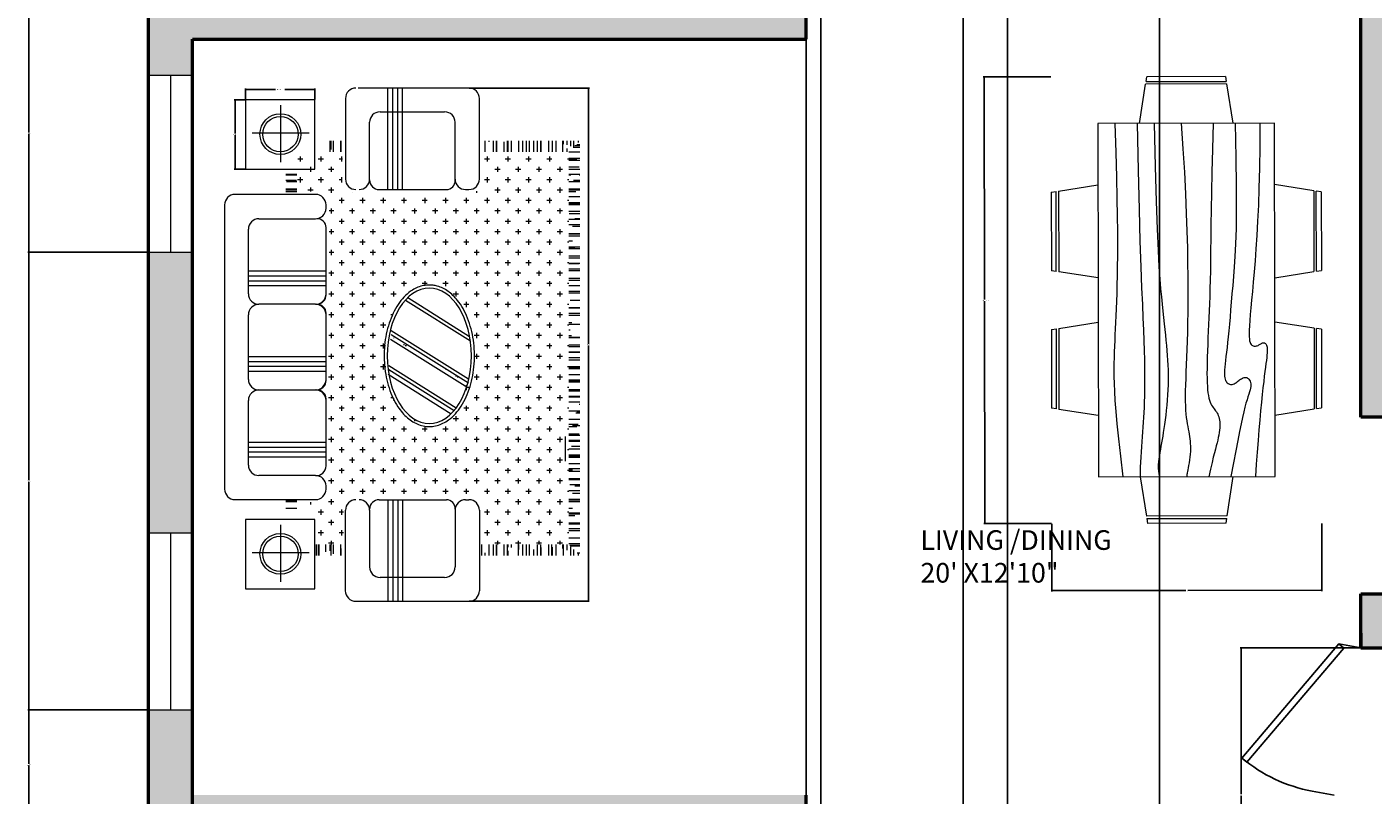
# Model space of a CAD drawing. Units: inches. Extents: x -23 to 411, y -22 to 507.
# Tile 2 of 5: x -23 to 252, y 159 to 315. Entities that reach past the tile are written whole.
import ezdxf

# ---------------------------------------------------------------- set-up
doc = ezdxf.new("R2010")
doc.units = ezdxf.units.IN
doc.header["$MEASUREMENT"] = 0
for name, color, linetype, lineweight in [('A-ANNO-DIMS', 2, 'Continuous', 18), ('A-AREA-IDEN', 7, 'Continuous', 25), ('A-FURN-PATT', 7, 'Continuous', 13), ('A-WALL', 7, 'Continuous', 50), ('doors', 40, 'Continuous', 25), ('furniture', 220, 'Continuous', 18), ('window', 30, 'Continuous', 18)]:
    doc.layers.add(name, color=color, linetype=linetype, lineweight=lineweight)
doc.layers.add('A-WALL-PATT', color=179, linetype='Continuous', lineweight=13, true_color=0x161b4b)
doc.styles.get("Standard").update_dxf_attribs({"font": 'arial.ttf'})
doc.dimstyles.get("Standard").update_dxf_attribs({"dimtxt": 0.18, "dimasz": 0.18, "dimexe": 0.18, "dimexo": 0.0625, "dimgap": 0.09, "dimtad": 0, "dimtih": 1, "dimtoh": 1, "dimdec": 4, "dimzin": 0, "dimdsep": 46, "dimtxsty": 'Standard', "dimcen": 0.09, "dimadec": 0, "dimazin": 0, "dimtfac": 1, "dimtdec": 4, "dimtofl": 0, "dimtmove": 0, "dimatfit": 3, "dimfxl": 1, "dimtolj": 1, "dimtzin": 0, "dimarcsym": 0})

# ---------------------------------------------------------------- blocks, each defined once
blk = doc.blocks.new('*U6')
for p, q in [((0, 0), (0, -6)), ((40, 0), (40, -6))]:
    blk.add_line(p, q)
blk.add_lwpolyline([(0, 0), (34.64, 20), (35.52, 18.48), (0.87, -1.52)], close=True)
blk.add_arc((0, 0), 40, 0, 30)
blk = doc.blocks.new('Dining Set - 36 x 72 in.')
for p, q in [((-22, 27.5), (-22.1562, 26.50042)), ((-22, 27.5), (-6, 27.5)), ((-5.8437, 26.49966), (-6, 27.5)), ((6, 27.5), (5.8438, 26.50042)), ((6, 27.5), (22, 27.5)), ((22.1563, 26.49966), (22, 27.5)), ((-22.2343, 26.00059), (-23.4847, 17.99762)), ((-22.2304, 26), (-5.7608, 26)), ((-5.8416, 26.5), (-22.1534, 26.5)), ((-4.5152, 17.99762), (-5.7655, 25.99926)), ((5.7657, 26.00059), (4.5153, 17.99762)), ((5.7696, 26), (22.2392, 26)), ((22.1584, 26.5), (5.8466, 26.5)), ((23.4848, 17.99762), (22.2345, 25.99926)), ((36, 18), (-36, 18)), ((-36, 18), (-36, -18)), ((36, -18), (36, 18)), ((-44.0006, 8.23428), (-35.9976, 9.48474)), ((-44, 8.23041), (-44, -8.23915)), ((44.0006, 8.23428), (35.9976, 9.48474)), ((44, 8.23041), (44, -8.23915)), ((-45.5, 8), (-44.5004, 8.15617)), ((-45.5, 8), (-45.5, -8)), ((-44.5, -8.15843), (-44.5, 8.15338)), ((44.5, -8.15843), (44.5, 8.15338)), ((45.5, 8), (44.5005, 8.15617)), ((45.5, 8), (45.5, -8)), ((-44.4997, -8.15631), (-45.5, -8)), ((44.4997, -8.15631), (45.5, -8)), ((-35.9976, -9.48476), (-43.9993, -8.2345)), ((35.9976, -9.48476), (43.9993, -8.2345)), ((-36, -18), (36, -18)), ((-22.2343, -26.0006), (-23.4847, -17.99762)), ((-4.5152, -17.99762), (-5.7655, -25.99928)), ((5.7657, -26.0006), (4.5153, -17.99762)), ((23.4848, -17.99762), (22.2345, -25.99928)), ((-22.2304, -26), (-5.7608, -26)), ((-22, -27.5), (-22.1562, -26.50044)), ((-5.8416, -26.5), (-22.1534, -26.5)), ((-5.8437, -26.49967), (-6, -27.5)), ((5.7696, -26), (22.2392, -26)), ((6, -27.5), (5.8438, -26.50044)), ((22.1584, -26.5), (5.8466, -26.5)), ((22.1563, -26.49967), (22, -27.5)), ((-22, -27.5), (-6, -27.5)), ((6, -27.5), (22, -27.5))]:
    blk.add_line(p, q)
for points in [[(-36, 15), (-31.1772, 14.97754), (-26.8079, 14.91406), (-22.8538, 14.81543), (-19.276, 14.6875), (-16.0362, 14.53613), (-13.0957, 14.36718), (-10.4159, 14.18652), (-7.9583, 14), (-5.6904, 13.81315), (-3.6035, 13.63021), (-1.6954, 13.45508), (0.0365, 13.29166), (1.5945, 13.14388), (2.9811, 13.01562), (4.1988, 12.9108), (5.25, 12.83333), (6.1393, 12.78613), (6.8802, 12.76823), (7.4883, 12.77767), (7.9792, 12.8125), (8.3685, 12.87077), (8.6719, 12.95052), (8.9049, 13.0498), (9.0833, 13.16666), (9.2205, 13.29899), (9.3216, 13.44401), (9.3895, 13.59879), (9.4271, 13.76041), (9.4373, 13.92594), (9.4232, 14.09245), (9.3875, 14.257), (9.3333, 14.41666), (9.2638, 14.56917), (9.1836, 14.71484), (9.0975, 14.85465), (9.0104, 14.98958), (8.9272, 15.1206), (8.8529, 15.2487), (8.7922, 15.37483), (8.75, 15.5), (8.7305, 15.62467), (8.7344, 15.74739), (8.7617, 15.86621), (8.8125, 15.97916), (8.8867, 16.08431), (8.9844, 16.17968), (9.1055, 16.26334), (9.25, 16.33333), (9.4189, 16.38802), (9.6172, 16.42708), (9.8506, 16.45052), (10.125, 16.45833), (10.4463, 16.45052), (10.8203, 16.42708), (11.2529, 16.38802), (11.75, 16.33333), (12.3184, 16.26318), (12.9694, 16.17838), (13.7151, 16.07991), (14.5677, 15.96875), (15.5395, 15.84586), (16.6426, 15.71224), (17.8893, 15.56884), (19.2917, 15.41666), (20.859, 15.25667), (22.5879, 15.08984), (24.4721, 14.91715), (26.5052, 14.73958), (28.6809, 14.5581), (30.9929, 14.3737), (33.4347, 14.18733), (36, 14)], [(-36, 10), (-28.9766, 10.14274), (-23.1725, 10.20442), (-18.4241, 10.19775), (-14.5677, 10.13541), (-11.4399, 10.03011), (-8.877, 9.89453), (-6.7154, 9.74137), (-4.7917, 9.58333), (-2.9698, 9.43082), (-1.2246, 9.28515), (0.4415, 9.14534), (2.026, 9.01041), (3.5266, 8.87939), (4.9408, 8.7513), (6.266, 8.62516), (7.5, 8.5), (8.6411, 8.37549), (9.6914, 8.2539), (10.6538, 8.13818), (11.5312, 8.03125), (12.3267, 7.93603), (13.043, 7.85547), (13.6831, 7.79248), (14.25, 7.75), (14.7471, 7.7303), (15.1797, 7.73307), (15.5537, 7.75732), (15.875, 7.80208), (16.1494, 7.86637), (16.3828, 7.94922), (16.5811, 8.04964), (16.75, 8.16666), (16.8944, 8.29915), (17.0143, 8.44531), (17.1089, 8.60319), (17.1771, 8.77083), (17.218, 8.94629), (17.2305, 9.1276), (17.2137, 9.31282), (17.1667, 9.5), (17.0895, 9.6875), (16.987, 9.875), (16.8649, 10.0625), (16.7292, 10.25), (16.5856, 10.4375), (16.4401, 10.625), (16.2985, 10.8125), (16.1667, 11), (16.05, 11.18733), (15.9518, 11.3737), (15.8752, 11.5581), (15.8229, 11.73958), (15.798, 11.91715), (15.8034, 12.08984), (15.842, 12.25667), (15.9167, 12.41666), (16.0295, 12.56836), (16.1784, 12.70833), (16.3605, 12.83268), (16.5729, 12.9375), (16.8127, 13.01888), (17.0768, 13.07291), (17.3625, 13.0957), (17.6667, 13.08333), (17.9894, 13.03312), (18.3418, 12.94726), (18.7382, 12.82918), (19.1927, 12.68229), (19.7195, 12.51001), (20.3327, 12.31575), (21.0465, 12.10294), (21.875, 11.875), (22.8357, 11.63354), (23.959, 11.37304), (25.2786, 11.08618), (26.8282, 10.76562), (28.6414, 10.40405), (30.752, 9.99414), (33.1936, 9.52856), (36, 9)], [(-36, 5.5), (-30.7157, 5.3348), (-26.069, 5.20963), (-21.9946, 5.11767), (-18.4271, 5.05208), (-15.3009, 5.00602), (-12.5508, 4.97265), (-10.1112, 4.94515), (-7.9167, 4.91666), (-5.909, 4.88167), (-4.0586, 4.83984), (-2.3429, 4.79215), (-0.7396, 4.73958), (0.7739, 4.6831), (2.22, 4.6237), (3.6213, 4.56233), (5, 4.5), (6.373, 4.43782), (7.7344, 4.3776), (9.0723, 4.32129), (10.375, 4.27083), (11.6309, 4.22819), (12.8281, 4.19531), (13.9551, 4.17415), (15, 4.16666), (15.954, 4.17448), (16.819, 4.19791), (17.6001, 4.23698), (18.3021, 4.29166), (18.9299, 4.36198), (19.4883, 4.44791), (19.9823, 4.54948), (20.4167, 4.66666), (20.7969, 4.79899), (21.1302, 4.94401), (21.4245, 5.09879), (21.6875, 5.26041), (21.9271, 5.42594), (22.1511, 5.59245), (22.3672, 5.757), (22.5834, 5.91666), (22.8065, 6.06868), (23.0404, 6.21093), (23.2879, 6.34147), (23.5521, 6.45833), (23.8358, 6.55957), (24.142, 6.64323), (24.4735, 6.70735), (24.8334, 6.75), (25.2235, 6.76969), (25.642, 6.76692), (26.0858, 6.74267), (26.5521, 6.69791), (27.0379, 6.63362), (27.5404, 6.55078), (28.0565, 6.45036), (28.5834, 6.33333), (29.1242, 6.19987), (29.7071, 6.04687), (30.3661, 5.87044), (31.1354, 5.66666), (32.0493, 5.43164), (33.142, 5.16146), (34.4475, 4.85221), (36, 4.5)], [(-36, -1), (-30.7915, -0.6591), (-26.0195, -0.38216), (-21.6519, -0.16284), (-17.6563, 0.00521), (-14.0005, 0.12833), (-10.6523, 0.21289), (-7.5796, 0.26522), (-4.75, 0.29166), (-2.134, 0.29793), (0.2878, 0.28711), (2.5317, 0.26163), (4.6146, 0.22396), (6.5529, 0.17651), (8.3633, 0.12174), (10.0623, 0.06209), (11.6667, 0), (13.1899, -0.06201), (14.6341, -0.1211), (15.9982, -0.17432), (17.2813, -0.21875), (18.4823, -0.25147), (19.6003, -0.26953), (20.6343, -0.27002), (21.5834, -0.25), (22.4481, -0.20768), (23.2357, -0.14584), (23.9549, -0.06836), (24.6146, 0.02083), (25.2235, 0.11784), (25.7904, 0.21875), (26.3241, 0.31966), (26.8334, 0.41666), (27.3265, 0.50618), (27.8099, 0.58593), (28.2894, 0.65397), (28.7709, 0.70833), (29.2601, 0.74707), (29.763, 0.76823), (30.2855, 0.76985), (30.8334, 0.75), (31.4088, 0.70784), (31.9994, 0.64713), (32.589, 0.57275), (33.1615, 0.48958), (33.7008, 0.4025), (34.1908, 0.3164), (34.6153, 0.23616), (34.9584, 0.16666), (35.2099, 0.11165), (35.3848, 0.07031), (35.504, 0.04069), (35.5886, 0.02083), (35.6594, 0.00879), (35.7377, 0.0026), (35.8442, 0.00032), (36, 0)], [(-36, -6.5), (-27.1843, -6.31267), (-20.084, -6.1263), (-14.469, -5.9419), (-10.1094, -5.76042), (-6.7752, -5.58285), (-4.2363, -5.41016), (-2.2629, -5.24333), (-0.625, -5.08334), (0.8708, -4.93099), (2.2715, -4.78646), (3.5872, -4.64974), (4.8281, -4.52084), (6.0046, -4.39974), (7.127, -4.28646), (8.2053, -4.18099), (9.25, -4.08334), (10.2705, -3.99382), (11.2734, -3.91407), (12.2647, -3.84603), (13.25, -3.79167), (14.2354, -3.75293), (15.2266, -3.73177), (16.2295, -3.73015), (17.25, -3.75), (18.2912, -3.79248), (19.3451, -3.85547), (20.4009, -3.93604), (21.4479, -4.03125), (22.4754, -4.13819), (23.4727, -4.25391), (24.4289, -4.37549), (25.3334, -4.5), (26.1785, -4.62492), (26.9694, -4.74935), (27.7145, -4.87281), (28.4219, -4.99479), (29.1, -5.11483), (29.7572, -5.23242), (30.4016, -5.34709), (31.0417, -5.45834), (31.6837, -5.56437), (32.3262, -5.65821), (32.9658, -5.73153), (33.599, -5.77604), (34.2224, -5.78345), (34.8327, -5.74545), (35.4264, -5.65373), (36, -5.5)], [(-36, -10), (-26.4022, -9.81299), (-18.4675, -9.62891), (-11.9839, -9.45069), (-6.7396, -9.28125), (-2.5226, -9.12354), (0.8789, -8.98047), (3.6769, -8.85498), (6.0833, -8.75), (8.2767, -8.66765), (10.3021, -8.60677), (12.1712, -8.56543), (13.8958, -8.54167), (15.4876, -8.53353), (16.9583, -8.53907), (18.3197, -8.55632), (19.5834, -8.58334), (20.7616, -8.61841), (21.8685, -8.66081), (22.9188, -8.71004), (23.9271, -8.76563), (24.9081, -8.82707), (25.8763, -8.89388), (26.8465, -8.96558), (27.8334, -9.04167), (28.8474, -9.12118), (29.8828, -9.20117), (30.93, -9.27824), (31.9792, -9.34896), (33.0205, -9.40991), (34.0443, -9.45768), (35.0407, -9.48885), (36, -9.5)], [(-36, -14.5), (-30.0881, -14.33513), (-25.0332, -14.21224), (-20.7312, -14.12647), (-17.0781, -14.07292), (-13.97, -14.04671), (-11.3027, -14.04297), (-8.9724, -14.05681), (-6.875, -14.08334), (-4.9224, -14.11833), (-3.0905, -14.16016), (-1.3709, -14.20785), (0.2448, -14.26042), (1.7647, -14.3169), (3.1973, -14.3763), (4.5507, -14.43767), (5.8333, -14.5), (7.0554, -14.5621), (8.235, -14.62175), (9.3922, -14.67652), (10.5469, -14.72396), (11.7192, -14.76164), (12.929, -14.78711), (14.1965, -14.79794), (15.5417, -14.79167), (16.9933, -14.76424), (18.6152, -14.70508), (20.4804, -14.60197), (22.6615, -14.44271), (25.2312, -14.21509), (28.2624, -13.9069), (31.8277, -13.50594), (36, -13)]]:
    blk.add_lwpolyline(points)
blk = doc.blocks.new('WIN-36IN')
for p, q in [((9, 36), (0, 36)), ((0, 36), (0, 0)), ((4.5, 0), (4.5, 36)), ((9, 0), (9, 36)), ((0, 0), (9, 0)), ((0, 0), (4.5, 0))]:
    blk.add_line(p, q)
blk = doc.blocks.new('END-TABLE-LAMP')
for p, q in [((14.11, 14.11), (0, 14.11)), ((0, 14.11), (0, 0)), ((14.11, 0), (14.11, 14.11)), ((7.16, 1.4), (7.16, 13.04)), ((12.97, 7.3), (1.33, 7.3)), ((0, 0), (14.11, 0))]:
    blk.add_line(p, q)
for radius in [4.16, 3.6]:
    blk.add_circle((7.1, 7.11), radius)
blk = doc.blocks.new('*D20')
at = {"layer": 'A-ANNO-DIMS', "color": 0, "lineweight": -2, "transparency": 16777216}
for p, q in [((21.97, 300.62), (21.97, 302.85)), ((22.15, 302.67), (28.06, 302.67)), ((35.89, 302.67), (29.98, 302.67)), ((36.07, 300.62), (36.07, 302.85))]:
    blk.add_line(p, q, dxfattribs=at)
at = {"layer": 'A-ANNO-DIMS', "color": 0, "transparency": 16777216}
for points in [[(22.15, 302.7), (22.15, 302.64), (21.97, 302.67)], [(35.89, 302.7), (35.89, 302.64), (36.07, 302.67)]]:
    blk.add_solid(points, dxfattribs=at)
at = {"layer": 'Defpoints', "color": 0, "transparency": 16777216}
for p in [(36.07, 302.67), (21.97, 300.55), (36.07, 300.55)]:
    blk.add_point(p, dxfattribs=at)
at = {"layer": 'A-ANNO-DIMS', "color": 0, "transparency": 16777216, "insert": (29.02, 302.67), "char_height": 0.18, "attachment_point": 5}
blk.add_mtext('\\A1;TABLE 14 TYP.', dxfattribs=at)
blk = doc.blocks.new('*D21')
at = {"layer": 'A-ANNO-DIMS', "color": 0, "lineweight": -2, "transparency": 16777216}
for p, q in [((21.9, 300.55), (19.67, 300.55)), ((19.85, 300.37), (19.85, 293.68)), ((19.85, 286.63), (19.85, 293.32)), ((21.9, 286.45), (19.67, 286.45))]:
    blk.add_line(p, q, dxfattribs=at)
at = {"layer": 'A-ANNO-DIMS', "color": 0, "transparency": 16777216}
for points in [[(19.82, 300.37), (19.88, 300.37), (19.85, 300.55)], [(19.82, 286.63), (19.88, 286.63), (19.85, 286.45)]]:
    blk.add_solid(points, dxfattribs=at)
at = {"layer": 'Defpoints', "color": 0, "transparency": 16777216}
for p in [(19.85, 300.55), (21.97, 300.55), (21.97, 286.45)]:
    blk.add_point(p, dxfattribs=at)
at = {"layer": 'A-ANNO-DIMS', "color": 0, "transparency": 16777216, "insert": (19.85, 293.5), "char_height": 0.18, "attachment_point": 5}
blk.add_mtext('\\A1;14 TYP.', dxfattribs=at)
blk = doc.blocks.new('*D26')
at = {"layer": 'A-ANNO-DIMS', "color": 0, "lineweight": -2, "transparency": 16777216}
for p, q in [((186.01, 305.22), (172.25, 305.2)), ((172.43, 305.02), (172.5, 259.88)), ((172.57, 214.38), (172.5, 259.51)), ((186.15, 214.22), (172.39, 214.2))]:
    blk.add_line(p, q, dxfattribs=at)
at = {"layer": 'A-ANNO-DIMS', "color": 0, "transparency": 16777216}
for points in [[(172.46, 305.02), (172.4, 305.02), (172.43, 305.2)], [(172.6, 214.38), (172.54, 214.38), (172.57, 214.2)]]:
    blk.add_solid(points, dxfattribs=at)
at = {"layer": 'Defpoints', "color": 0, "transparency": 16777216}
for p in [(186.08, 305.22), (172.57, 214.2), (186.22, 214.22)]:
    blk.add_point(p, dxfattribs=at)
at = {"layer": 'A-ANNO-DIMS', "color": 0, "transparency": 16777216, "insert": (172.5, 259.7), "char_height": 0.18, "attachment_point": 5}
blk.add_mtext('\\A1;DINING SET 91', dxfattribs=at)
blk = doc.blocks.new('*D27')
at = {"layer": 'A-ANNO-DIMS', "color": 0, "lineweight": -2, "transparency": 16777216}
for p, q in [((186.22, 214.16), (186.24, 200.39)), ((241.22, 214.24), (241.24, 200.47)), ((186.42, 200.57), (213.52, 200.61)), ((241.06, 200.65), (213.96, 200.61))]:
    blk.add_line(p, q, dxfattribs=at)
at = {"layer": 'A-ANNO-DIMS', "color": 0, "transparency": 16777216}
for points in [[(186.42, 200.6), (186.42, 200.54), (186.24, 200.57)], [(241.06, 200.68), (241.06, 200.62), (241.24, 200.65)]]:
    blk.add_solid(points, dxfattribs=at)
at = {"layer": 'Defpoints', "color": 0, "transparency": 16777216}
for p in [(186.22, 214.22), (241.22, 214.3), (241.24, 200.65)]:
    blk.add_point(p, dxfattribs=at)
at = {"layer": 'A-ANNO-DIMS', "color": 0, "transparency": 16777216, "insert": (213.74, 200.61), "char_height": 0.18, "attachment_point": 5}
blk.add_mtext('\\A1;55', dxfattribs=at)
blk = doc.blocks.new('*D40')
at = {"layer": 'A-ANNO-DIMS', "color": 0, "lineweight": -2, "transparency": 16777216}
for p, q in [((2.11, 176.25), (-22.38, 176.25)), ((-22.2, 176.07), (-22.2, 165.26)), ((-22.2, 154.08), (-22.2, 164.89)), ((11.11, 153.9), (-22.38, 153.9))]:
    blk.add_line(p, q, dxfattribs=at)
at = {"layer": 'A-ANNO-DIMS', "color": 0, "transparency": 16777216}
for points in [[(-22.23, 176.07), (-22.17, 176.07), (-22.2, 176.25)], [(-22.23, 154.08), (-22.17, 154.08), (-22.2, 153.9)]]:
    blk.add_solid(points, dxfattribs=at)
at = {"layer": 'Defpoints', "color": 0, "transparency": 16777216}
for p in [(-22.2, 176.25), (2.17, 176.25), (11.17, 153.9)]:
    blk.add_point(p, dxfattribs=at)
at = {"layer": 'A-ANNO-DIMS', "color": 0, "transparency": 16777216, "insert": (-22.2, 165.08), "char_height": 0.18, "attachment_point": 5}
blk.add_mtext('\\A1;22.358', dxfattribs=at)
blk = doc.blocks.new('*D41')
at = {"layer": 'A-ANNO-DIMS', "color": 0, "lineweight": -2, "transparency": 16777216}
for p, q in [((2.11, 269.51), (-22.38, 269.51)), ((-22.2, 269.33), (-22.2, 223.06)), ((-22.2, 176.43), (-22.2, 222.7)), ((2.11, 176.25), (-22.38, 176.25))]:
    blk.add_line(p, q, dxfattribs=at)
at = {"layer": 'A-ANNO-DIMS', "color": 0, "transparency": 16777216}
for points in [[(-22.23, 269.33), (-22.17, 269.33), (-22.2, 269.51)], [(-22.23, 176.43), (-22.17, 176.43), (-22.2, 176.25)]]:
    blk.add_solid(points, dxfattribs=at)
at = {"layer": 'Defpoints', "color": 0, "transparency": 16777216}
for p in [(-22.2, 269.51), (2.17, 269.51), (2.17, 176.25)]:
    blk.add_point(p, dxfattribs=at)
at = {"layer": 'A-ANNO-DIMS', "color": 0, "transparency": 16777216, "insert": (-22.2, 222.88), "char_height": 0.18, "attachment_point": 5}
blk.add_mtext('\\A1;93.25', dxfattribs=at)
blk = doc.blocks.new('*D42')
at = {"layer": 'A-ANNO-DIMS', "color": 0, "lineweight": -2, "transparency": 16777216}
for p, q in [((11.11, 317.9), (-22.38, 317.9)), ((-22.2, 317.72), (-22.2, 293.88)), ((-22.2, 269.69), (-22.2, 293.52)), ((2.11, 269.51), (-22.38, 269.51))]:
    blk.add_line(p, q, dxfattribs=at)
at = {"layer": 'A-ANNO-DIMS', "color": 0, "transparency": 16777216}
for points in [[(-22.23, 317.72), (-22.17, 317.72), (-22.2, 317.9)], [(-22.23, 269.69), (-22.17, 269.69), (-22.2, 269.51)]]:
    blk.add_solid(points, dxfattribs=at)
at = {"layer": 'Defpoints', "color": 0, "transparency": 16777216}
for p in [(-22.2, 317.9), (11.17, 317.9), (2.17, 269.51)]:
    blk.add_point(p, dxfattribs=at)
at = {"layer": 'A-ANNO-DIMS', "color": 0, "transparency": 16777216, "insert": (-22.2, 293.7), "char_height": 0.18, "attachment_point": 5}
blk.add_mtext('\\A1;48.39', dxfattribs=at)
blk = doc.blocks.new('*D45')
at = {"layer": 'A-ANNO-DIMS', "color": 0, "lineweight": -2, "transparency": 16777216}
for p, q in [((136.17, 107.96), (136.17, 507.45)), ((177.17, 107.96), (177.17, 507.45)), ((136.35, 507.27), (156.47, 507.27)), ((176.99, 507.27), (156.88, 507.27))]:
    blk.add_line(p, q, dxfattribs=at)
at = {"layer": 'A-ANNO-DIMS', "color": 0, "transparency": 16777216}
for points in [[(136.35, 507.3), (136.35, 507.24), (136.17, 507.27)], [(176.99, 507.3), (176.99, 507.24), (177.17, 507.27)]]:
    blk.add_solid(points, dxfattribs=at)
at = {"layer": 'Defpoints', "color": 0, "transparency": 16777216}
for p in [(177.17, 507.27), (136.17, 107.9), (177.17, 107.9)]:
    blk.add_point(p, dxfattribs=at)
at = {"layer": 'A-ANNO-DIMS', "color": 0, "transparency": 16777216, "insert": (156.67, 507.27), "char_height": 0.18, "attachment_point": 5}
blk.add_mtext('\\A1;41', dxfattribs=at)
blk = doc.blocks.new('*D46')
at = {"layer": 'A-ANNO-DIMS', "color": 0, "lineweight": -2, "transparency": 16777216}
for p, q in [((177.17, 107.96), (177.17, 507.45)), ((208.17, 107.96), (208.17, 507.45)), ((177.35, 507.27), (192.47, 507.27)), ((207.99, 507.27), (192.88, 507.27))]:
    blk.add_line(p, q, dxfattribs=at)
at = {"layer": 'A-ANNO-DIMS', "color": 0, "transparency": 16777216}
for points in [[(177.35, 507.3), (177.35, 507.24), (177.17, 507.27)], [(207.99, 507.3), (207.99, 507.24), (208.17, 507.27)]]:
    blk.add_solid(points, dxfattribs=at)
at = {"layer": 'Defpoints', "color": 0, "transparency": 16777216}
for p in [(208.17, 507.27), (177.17, 107.9), (208.17, 107.9)]:
    blk.add_point(p, dxfattribs=at)
at = {"layer": 'A-ANNO-DIMS', "color": 0, "transparency": 16777216, "insert": (192.67, 507.27), "char_height": 0.18, "attachment_point": 5}
blk.add_mtext('\\A1;31', dxfattribs=at)
blk = doc.blocks.new('*D50')
at = {"layer": 'A-ANNO-DIMS', "color": 0, "lineweight": -2, "transparency": 16777216}
for p, q in [((139.17, 372.83), (139.17, -21.66)), ((168.17, 372.83), (168.17, -21.66)), ((139.35, -21.48), (153.45, -21.48)), ((167.99, -21.48), (153.9, -21.48))]:
    blk.add_line(p, q, dxfattribs=at)
at = {"layer": 'A-ANNO-DIMS', "color": 0, "transparency": 16777216}
for points in [[(139.35, -21.45), (139.35, -21.51), (139.17, -21.48)], [(167.99, -21.45), (167.99, -21.51), (168.17, -21.48)]]:
    blk.add_solid(points, dxfattribs=at)
at = {"layer": 'Defpoints', "color": 0, "transparency": 16777216}
for p in [(139.17, 372.9), (168.17, 372.9), (168.17, -21.48)]:
    blk.add_point(p, dxfattribs=at)
at = {"layer": 'A-ANNO-DIMS', "color": 0, "transparency": 16777216, "insert": (153.67, -21.48), "char_height": 0.18, "attachment_point": 5}
blk.add_mtext('\\A1;29', dxfattribs=at)
blk = doc.blocks.new('*D52')
at = {"layer": 'A-ANNO-DIMS', "color": 0, "lineweight": -2, "transparency": 16777216}
for p, q in [((249.11, 188.9), (224.62, 188.9)), ((224.8, 188.72), (224.8, 159.08)), ((224.8, 129.08), (224.8, 158.72)), ((249.11, 128.9), (224.62, 128.9))]:
    blk.add_line(p, q, dxfattribs=at)
at = {"layer": 'A-ANNO-DIMS', "color": 0, "transparency": 16777216}
for points in [[(224.77, 188.72), (224.83, 188.72), (224.8, 188.9)], [(224.77, 129.08), (224.83, 129.08), (224.8, 128.9)]]:
    blk.add_solid(points, dxfattribs=at)
at = {"layer": 'Defpoints', "color": 0, "transparency": 16777216}
for p in [(224.8, 188.9), (249.17, 188.9), (249.17, 128.9)]:
    blk.add_point(p, dxfattribs=at)
at = {"layer": 'A-ANNO-DIMS', "color": 0, "transparency": 16777216, "insert": (224.8, 158.9), "char_height": 0.18, "attachment_point": 5}
blk.add_mtext('\\A1;60', dxfattribs=at)
blk = doc.blocks.new('*D68')
at = {"layer": 'A-ANNO-DIMS', "color": 0, "lineweight": -2, "transparency": 16777216}
for p, q in [((67.54, 302.95), (92.03, 302.94)), ((91.85, 302.76), (91.83, 250.84)), ((91.81, 198.55), (91.83, 250.47)), ((67.5, 198.38), (91.99, 198.37))]:
    blk.add_line(p, q, dxfattribs=at)
at = {"layer": 'A-ANNO-DIMS', "color": 0, "transparency": 16777216}
for points in [[(91.82, 302.76), (91.88, 302.76), (91.85, 302.94)], [(91.78, 198.55), (91.84, 198.55), (91.81, 198.37)]]:
    blk.add_solid(points, dxfattribs=at)
at = {"layer": 'Defpoints', "color": 0, "transparency": 16777216}
for p in [(67.47, 302.95), (67.43, 198.38), (91.81, 198.37)]:
    blk.add_point(p, dxfattribs=at)
at = {"layer": 'A-ANNO-DIMS', "color": 0, "transparency": 16777216, "insert": (91.83, 250.66), "char_height": 0.18, "attachment_point": 5}
blk.add_mtext('\\A1;104.57', dxfattribs=at)

msp = doc.modelspace()

# ---------------------------------------------------------------- hatches: boundary and pattern name
at = {"layer": 'A-FURN-PATT'}
h = msp.add_hatch(dxfattribs=at)
h.set_pattern_fill('AR-RROOF', color=256, scale=2.507942, angle=630, style=0)
h.set_pattern_definition([(180, (280.6525, 566.2183), (-4.965726, 2.257148), [33.85722, -4.5143, 11.28574, -2.25715]), (180, (277.6505, 567.347), (2.257148, 3.002007), [6.771445, -0.74486, 13.54289, -1.69286]), (180, (279.5239, 568.1369), (-11.7371705, 1.5122893), [18.057185, -3.16001, 9.028593, -2.25715])])
h.paths.add_polyline_path([(30.1745, 217.1169), (30.1745, 219.099), (32.4316, 219.099), (32.4316, 217.1169)])
h.paths.add_polyline_path([(87.8143, 209.9474), (87.8143, 289.9454), (90.0715, 292.2026), (90.0715, 207.6903)])
h.paths.add_polyline_path([(30.1745, 281.2713), (30.1745, 286.5075), (32.4316, 286.2113), (32.4316, 281.2713)])
h = msp.add_hatch(dxfattribs=at)
h.set_pattern_fill('AR-RROOF', color=256, scale=2.507942, angle=540, style=0)
h.set_pattern_definition([(270, (280.6525, 566.2183), (-2.257148, -4.965726), [33.85722, -4.5143, 11.28574, -2.25715]), (270, (279.524, 563.2163), (-3.002007, 2.257148), [6.771445, -0.74486, 13.54289, -1.69286]), (270, (278.7339, 565.0897), (-1.5122893, -11.7371705), [18.057185, -3.16001, 9.028593, -2.25715])])
h.paths.add_polyline_path([(36.0733, 207.6903), (36.0733, 209.9474), (42.3249, 209.9474), (42.3249, 207.6903)])
h.paths.add_polyline_path([(69.6111, 207.6903), (69.6111, 209.9474), (87.8143, 209.9474), (90.0715, 207.6903)])
h.paths.add_polyline_path([(69.6111, 289.9454), (69.6111, 292.2026), (90.0715, 292.2026), (87.8143, 289.9454)])
h.paths.add_polyline_path([(38.8085, 289.9454), (39.1053, 292.2026), (42.3249, 292.2026), (42.3249, 289.9454)])
h = msp.add_hatch(dxfattribs=at)
h.set_pattern_fill('CROSS', color=256, scale=9.404784, angle=540, style=0)
h.set_pattern_definition([(270, (280.6525, 566.2183), (-2.116076, -2.116076), [1.058038, -3.174115]), (180, (281.1815, 565.6893), (-2.116076, 2.116076), [1.058038, -3.174115])])
h.paths.add_polyline_path([(70.3061, 209.9474), (70.0785, 217.8597), (69.9429, 219.4877), (43.5045, 219.6233), (41.8775, 218.6737), (41.9713, 209.9474), (36.0733, 209.9474), (36.0733, 217.1169), (32.4316, 217.1169), (32.4316, 218.5071), (38.7591, 218.6737), (39.0303, 280.3994), (38.0812, 281.8916), (32.4316, 281.8131), (32.4316, 287.1803), (32.8314, 289.9454), (41.7554, 289.9454), (41.6063, 283.3839), (43.5045, 281.6203), (66.2822, 281.2133), (69.9429, 282.1629), (70.1938, 289.9454), (87.8143, 289.9454), (87.8143, 209.9474)])
h.paths.add_polyline_path([(67.7736, 246.4842), (67.638, 256.5231), (63.0283, 262.0851), (60.9945, 262.8991), (58.4185, 262.8991), (56.5203, 262.4921), (53.9443, 261.2712), (52.8596, 258.6936), (51.3682, 255.7091), (50.6903, 252.4532), (50.2836, 248.5191), (51.775, 240.2438), (55.1645, 235.4956), (60.5878, 234.546), (63.7062, 236.0383), (66.4178, 239.9724)], flags=16)
edge = h.paths.add_edge_path(flags=0)
edge.add_line((66.5658, 243.1478), (51.7607, 252.0502))
edge.add_ellipse((74.6507, 248.5741), major_axis=(-16.3712, 16.3712), ratio=1, start_angle=35.87674, end_angle=36.365125, ccw=False)
edge.add_line((51.7912, 252.2451), (66.61, 243.3345))
edge.add_ellipse((44.0583, 248.5741), major_axis=(16.3712, 16.3712), ratio=1, start_angle=301.445378, end_angle=301.920237, ccw=False)
edge.add_line((66.5658, 243.1478), (66.5658, 243.1478))
edge.add_ellipse((51.6136, 246.7541), major_axis=(10.876, 10.876), ratio=0.9999999, start_angle=301.439889, end_angle=301.456246)
edge.add_line((66.5669, 243.1521), (66.5669, 243.1521))
edge.add_line((66.5669, 243.1521), (66.5669, 243.1521))
edge.add_line((66.5669, 243.1521), (66.5669, 243.1521))
edge.add_line((66.5669, 243.1521), (66.5669, 243.1521))
edge.add_line((66.5669, 243.1521), (66.5669, 243.1521))
edge.add_ellipse((51.6136, 246.7541), major_axis=(-10.876, 10.876), ratio=0.99999997, start_angle=211.439889, end_angle=211.456241, ccw=False)
at = {"layer": 'A-WALL-PATT'}
h = msp.add_hatch(color=256, dxfattribs=at)
h.dxf.hatch_style = 1
h.paths.add_polyline_path([(37.3453, 482.8972), (2.1746, 482.8972), (2.1746, 414.9823), (11.1746, 414.9823), (11.1746, 473.8972), (37.3453, 473.8972)])
h.paths.add_polyline_path([(149.2817, 482.8972), (73.3453, 482.8972), (73.3453, 473.8972), (131.1746, 473.8972), (131.1746, 356.8972), (136.1746, 356.8972), (136.1746, 372.8972), (139.1746, 372.8972), (139.1746, 377.8972), (136.1746, 377.8972), (136.1746, 473.8972), (149.2817, 473.8972)])
h.paths.add_polyline_path([(209.1361, 482.8972), (173.2817, 482.8972), (173.2817, 473.8972), (190.1746, 473.8972), (190.1746, 377.8972), (168.1746, 377.8972), (168.1746, 372.8972), (249.1746, 372.8972), (249.1746, 356.8972), (254.1746, 356.8972), (254.1746, 380.8972), (249.1746, 380.8972), (249.1746, 377.8972), (195.1746, 377.8972), (195.1746, 473.8972), (209.1361, 473.8972)])
h.paths.add_polyline_path([(309.9724, 482.8972), (233.1361, 482.8972), (233.1361, 473.8972), (249.1746, 473.8972), (249.1746, 409.8972), (254.1746, 409.8972), (254.1746, 473.8972), (309.9724, 473.8972)])
h.paths.add_polyline_path([(386.1746, 482.8972), (345.9724, 482.8972), (345.9724, 473.8972), (377.1746, 473.8972), (377.1746, 445.6454), (386.1746, 445.6454)])
h.paths.add_polyline_path([(386.1746, 409.6454), (377.1746, 409.6454), (377.1746, 317.8972), (254.1746, 317.8972), (254.1746, 320.8972), (249.1746, 320.8972), (249.1746, 317.8972), (249.1746, 235.8972), (254.1746, 235.8972), (254.1746, 312.8972), (377.1746, 312.8972), (377.1746, 281.3732), (386.1746, 281.3732)])
h.paths.add_polyline_path([(386.1746, 245.3732), (377.1746, 245.3732), (377.1746, 196.8972), (254.1746, 196.8972), (254.1746, 199.8972), (249.1746, 199.8972), (249.1746, 196.8972), (249.1746, 188.8972), (254.1746, 188.8972), (254.1746, 191.8972), (264.1746, 191.8972), (377.1746, 191.8972), (377.1746, 11.8972), (377.1746, 2.8972), (386.1746, 2.8972)])
h.paths.add_polyline_path([(254.1746, 128.8972), (249.1746, 128.8972), (249.1746, 11.8972), (206.9157, 11.8972), (206.9157, 2.8972), (254.1746, 2.8972)])
h.paths.add_polyline_path([(170.9157, 11.8972), (86.2116, 11.8972), (86.2116, 2.8972), (170.9157, 2.8972)])
h.paths.add_polyline_path([(136.1746, 114.8972), (131.1746, 114.8972), (131.1746, 11.8972), (136.1746, 11.8972)])
h.paths.add_polyline_path([(50.2116, 11.8972), (11.1746, 11.8972), (11.1746, 90.1201), (2.1746, 90.1201), (2.1746, 2.8972), (50.2116, 2.8972)])
h.paths.add_polyline_path([(11.1746, 176.2548), (2.1746, 176.2548), (2.1746, 126.1201), (11.1746, 126.1201)])
h.paths.add_polyline_path([(136.1746, 158.8972), (11.1746, 158.8972), (11.1746, 153.8972), (131.1746, 153.8972), (131.1746, 150.8972), (136.1746, 150.8972)])
h.paths.add_polyline_path([(11.1746, 269.5052), (2.1746, 269.5052), (2.1746, 212.2548), (11.1746, 212.2548)])
h.paths.add_polyline_path([(11.1746, 378.9823), (2.1746, 378.9823), (2.1746, 305.5052), (11.1746, 305.5052), (11.1746, 312.8972), (136.1746, 312.8972), (136.1746, 320.8972), (131.1746, 320.8972), (131.1746, 317.8972), (11.1746, 317.8972)])

# ---------------------------------------------------------------- linework, layer by layer
at = {"layer": 'A-FURN-PATT'}
msp.add_line((87.115, 226.9432), (87.115, 231.9432), dxfattribs=at)
at = {"layer": 'A-WALL'}
for p, q in [((136.1746, 312.8972), (136.1746, 320.8972)), ((249.1746, 235.8972), (249.1746, 320.8972)), ((11.1746, 312.8972), (136.1746, 312.8972)), ((11.1746, 158.8972), (11.1746, 312.8972)), ((254.1746, 235.8972), (249.1746, 235.8972)), ((249.1746, 188.8972), (249.1746, 199.8972)), ((249.1746, 196.8972), (249.1746, 199.8972)), ((249.1746, 199.8972), (254.1746, 199.8972)), ((11.1746, 11.8972), (11.1746, 191.8972)), ((249.1746, 191.8972), (249.1746, 188.8972)), ((249.1746, 188.8972), (254.1746, 188.8972)), ((136.1746, 150.8972), (136.1746, 158.8972))]:
    msp.add_line(p, q, dxfattribs=at)
msp.add_lwpolyline([(254.1746, 2.8972), (2.1746, 2.8972), (2.1746, 482.8972), (386.1746, 482.8972), (386.1746, 2.8972), (377.1746, 2.8972)], dxfattribs=at)
at = {"layer": 'furniture'}
for p, q in [((67.8939, 302.8902), (44.8729, 302.8902)), ((50.9699, 282.3193), (50.9699, 302.9501)), ((51.9653, 282.3193), (51.9653, 302.9501)), ((52.9607, 282.3193), (52.9607, 302.9501)), ((53.9561, 282.3193), (53.9561, 302.9501)), ((42.3249, 300.8131), (42.3249, 284.4078)), ((69.6111, 284.4078), (69.6111, 300.8131)), ((49.3672, 298.0958), (62.529, 298.0958)), ((47.2302, 284.4078), (47.2302, 295.9588)), ((64.6719, 284.2125), (64.666, 295.9588)), ((36.2295, 281.2713), (19.8241, 281.2713)), ((49.1729, 282.2708), (62.869, 282.2708)), ((66.7942, 282.2708), (67.4741, 282.2708)), ((17.6872, 279.1343), (17.6872, 221.2359)), ((38.3665, 278.4544), (38.3665, 279.2373)), ((24.6784, 276.3174), (36.2295, 276.3174)), ((38.3665, 260.8243), (38.3665, 274.5204)), ((22.5414, 261.0186), (22.5414, 274.1804)), ((38.3179, 265.6076), (22.5414, 265.6076)), ((38.3179, 264.6122), (22.5414, 264.6122)), ((38.3179, 263.6167), (22.5414, 263.6167)), ((38.3179, 262.6213), (22.5414, 262.6213)), ((36.2295, 258.8816), (24.6784, 258.8816)), ((54.5249, 259.7354), (67.7666, 251.4298)), ((55.0219, 260.2482), (67.6168, 252.3484)), ((22.5414, 243.5829), (22.5414, 256.7447)), ((38.3665, 243.3886), (38.3665, 257.0847)), ((51.6065, 253.5799), (67.383, 243.6844)), ((51.6065, 252.7552), (67.383, 242.8598)), ((51.4888, 251.8128), (67.2652, 241.9174)), ((38.3179, 248.1718), (22.5414, 248.1718)), ((38.3179, 247.1764), (22.5414, 247.1764)), ((38.3179, 246.181), (22.5414, 246.181)), ((38.3179, 245.1856), (22.5414, 245.1856)), ((51.0179, 244.6268), (63.8338, 236.5883)), ((51.1356, 246.3939), (64.8742, 237.7766)), ((51.1356, 245.5693), (64.4342, 237.228)), ((24.6784, 241.44), (36.2295, 241.44)), ((22.5414, 226.1413), (22.5414, 239.3031)), ((38.3665, 225.947), (38.3665, 239.643)), ((38.3179, 230.7302), (22.5414, 230.7302)), ((38.3179, 229.7348), (22.5414, 229.7348)), ((38.3179, 228.7394), (22.5414, 228.7394)), ((38.3179, 227.744), (22.5414, 227.744)), ((36.2295, 224.0043), (24.6784, 224.0043)), ((38.3665, 221.2359), (38.3665, 221.8673)), ((19.8241, 219.099), (36.2295, 219.099)), ((42.3249, 200.5189), (42.3249, 216.9243)), ((47.2302, 216.9243), (47.2302, 205.3732)), ((49.1729, 219.0612), (62.869, 219.0612)), ((50.9699, 219.0127), (50.9699, 198.3819)), ((51.9653, 219.0127), (51.9653, 198.3819)), ((52.9607, 219.0127), (52.9607, 198.3819)), ((53.9561, 219.0127), (53.9561, 198.3819)), ((64.6719, 217.1195), (64.666, 205.3732)), ((66.7942, 219.0612), (67.4741, 219.0612)), ((69.6111, 216.9243), (69.6111, 200.5189)), ((62.529, 203.2362), (49.3672, 203.2362)), ((44.4133, 198.3819), (67.4343, 198.3819))]:
    msp.add_line(p, q, dxfattribs=at)
for centre, radius, start, end in [((44.4619, 300.8131), 2.137, 90, 180), ((67.4741, 300.8131), 2.137, 0, 90), ((49.3672, 295.9588), 2.137, 90, 180), ((62.529, 295.9588), 2.137, 0, 90), ((44.4619, 284.4078), 2.137, 180, 270), ((45.0933, 284.4078), 2.137, 270, 0), ((49.1508, 284.1914), 1.9207, 179.370084, 270.65888), ((62.869, 284.0702), 1.7994, 270, 2.985951), ((66.7942, 284.4078), 2.137, 180, 270), ((67.4741, 284.4078), 2.137, 270, 0), ((19.8241, 279.1343), 2.137, 90, 180), ((36.2295, 279.1343), 2.137, 0, 90), ((36.2295, 278.4544), 2.137, 270, 0), ((24.6784, 274.1804), 2.137, 90, 180), ((36.567, 274.5204), 1.7994, 0, 92.985951), ((24.6784, 261.0186), 2.137, 180, 270), ((36.2295, 261.0186), 2.137, 270, 0), ((36.4459, 260.8023), 1.9207, 269.370084, 0.65888), ((24.6784, 256.7447), 2.137, 90, 180), ((36.2295, 256.7447), 2.137, 0, 90), ((36.567, 257.0847), 1.7994, 0, 92.985951), ((24.6784, 243.5829), 2.137, 180, 270), ((24.6784, 239.3031), 2.137, 90, 180), ((36.2295, 243.577), 2.137, 270, 0), ((36.2295, 239.3089), 2.137, 0, 90), ((36.4459, 243.3665), 1.9207, 269.370084, 0.65888), ((36.567, 239.643), 1.7994, 0, 92.985951), ((24.6784, 226.1413), 2.137, 180, 270), ((36.4286, 225.9319), 1.9379, 264.101853, 0.445527), ((36.2295, 221.8673), 2.137, 0, 90), ((19.8241, 221.2359), 2.137, 180, 270), ((36.2295, 221.2359), 2.137, 270, 0), ((44.4619, 216.9243), 2.137, 90, 180), ((45.0933, 216.9243), 2.137, 0, 90), ((49.1508, 217.1406), 1.9207, 89.34112, 180.629916), ((62.869, 217.2618), 1.7994, 357.014049, 90), ((66.7942, 216.9243), 2.137, 90, 180), ((67.4741, 216.9243), 2.137, 0, 90), ((49.3672, 205.3732), 2.137, 180, 270), ((62.529, 205.3732), 2.137, 270, 0), ((44.422, 200.5189), 2.137, 180, 270), ((67.4741, 200.5189), 2.137, 270, 0)]:
    msp.add_arc(centre, radius, start, end, dxfattribs=at)
at = {"layer": 'furniture', "extrusion": (0, 0, -1)}
msp.add_ellipse((59.4019, 248.3933), major_axis=(0, 13.7895), ratio=0.62186025, start_param=4.71238898, end_param=10.99557429, dxfattribs=at)
at = {"layer": 'furniture'}
msp.add_open_spline([(59.4019, 262.8097), (59.6745, 262.8097), (59.9471, 262.791), (60.4892, 262.7164), (60.7589, 262.6606), (61.4071, 262.4809), (61.7828, 262.3382), (62.5159, 261.983), (62.8734, 261.7705), (63.5651, 261.2808), (63.8994, 261.0036), (64.5407, 260.39), (64.8479, 260.0535), (65.5495, 259.1801), (65.9291, 258.6172), (66.6203, 257.402), (66.9318, 256.7496), (67.4797, 255.3737), (67.7161, 254.6501), (68.1083, 253.1518), (68.264, 252.3771), (68.4909, 250.7979), (68.5622, 249.9935), (68.6184, 248.3772), (68.6034, 247.5654), (68.4875, 245.957), (68.3866, 245.1604), (68.1015, 243.6044), (67.9172, 242.8451), (67.4698, 241.3847), (67.2066, 240.6837), (66.6073, 239.3594), (66.2713, 238.7361), (65.5338, 237.5849), (65.1323, 237.057), (64.2725, 236.1125), (63.8142, 235.6959), (62.9623, 235.0709), (62.5784, 234.8366), (61.7892, 234.4489), (61.3839, 234.2955), (60.56, 234.075), (60.1415, 234.0079), (59.3016, 233.9629), (58.8804, 233.9849), (58.0458, 234.1171), (57.6326, 234.2273), (56.8238, 234.5315), (56.4281, 234.7255), (55.6615, 235.1914), (55.2905, 235.4633), (54.5785, 236.0783), (54.2375, 236.4214), (53.5899, 237.1719), (53.2832, 237.5794), (52.6289, 238.5715), (52.2933, 239.174), (51.6912, 240.4557), (51.4248, 241.1347), (50.9671, 242.5513), (50.7759, 243.2888), (50.4729, 244.8025), (50.3612, 245.5788), (50.22, 247.1495), (50.1905, 247.9438), (50.2144, 249.5296), (50.2678, 250.3209), (50.4562, 251.8794), (50.5912, 252.6465), (50.9397, 254.1363), (51.1532, 254.8588), (51.6538, 256.2402), (51.9408, 256.899), (52.5823, 258.135), (52.9366, 258.7124), (53.7053, 259.7697), (54.1196, 260.2496), (54.9997, 261.0976), (55.4656, 261.4656), (56.3154, 261.9988), (56.6903, 262.1917), (57.4571, 262.502), (57.8488, 262.6194), (58.628, 262.7719), (59.0149, 262.8097), (59.4019, 262.8097)], degree=3, knots=[3.14159265, 3.14159265, 3.14159265, 3.14159265, 3.22691715, 3.22691715, 3.31224165, 3.31224165, 3.43426671, 3.43426671, 3.55629177, 3.55629177, 3.67831683, 3.67831683, 3.8003419, 3.8003419, 3.97157384, 3.97157384, 4.14280577, 4.14280577, 4.31403771, 4.31403771, 4.48526965, 4.48526965, 4.65650159, 4.65650159, 4.82773353, 4.82773353, 4.99896547, 4.99896547, 5.1701974, 5.1701974, 5.34142934, 5.34142934, 5.51266128, 5.51266128, 5.68389322, 5.68389322, 5.85512516, 5.85512516, 5.98669107, 5.98669107, 6.11825699, 6.11825699, 6.24982291, 6.24982291, 6.38138882, 6.38138882, 6.51295474, 6.51295474, 6.64452065, 6.64452065, 6.77608657, 6.77608657, 6.90765249, 6.90765249, 7.0392184, 7.0392184, 7.20701563, 7.20701563, 7.37481286, 7.37481286, 7.54261009, 7.54261009, 7.71040732, 7.71040732, 7.87820455, 7.87820455, 8.04600178, 8.04600178, 8.21379901, 8.21379901, 8.38159624, 8.38159624, 8.54939347, 8.54939347, 8.7171907, 8.7171907, 8.88498794, 8.88498794, 9.05278517, 9.05278517, 9.17820699, 9.17820699, 9.30362881, 9.30362881, 9.42477796, 9.42477796, 9.42477796, 9.42477796], dxfattribs=at)

# ---------------------------------------------------------------- block references
at = {"layer": 'doors', "xscale": -0.7622159057711965, "yscale": 0.7622159057711965, "zscale": 0.7622159057711965, "rotation": 79.72827920711865}
msp.add_blockref('*U6', (244.6746, 189.7127), dxfattribs=at)
at = {"layer": 'furniture', "rotation": 270.0891389700014}
msp.add_blockref('Dining Set - 36 x 72 in.', (213.6466, 259.7613), dxfattribs=at)
at = {"layer": 'furniture'}
for p in [(21.966, 286.446), (21.966, 200.939)]:
    msp.add_blockref('END-TABLE-LAMP', p, dxfattribs=at)
at = {"layer": 'window', "rotation": 180}
for p in [(11.1741, 305.5054), (11.1741, 212.255)]:
    msp.add_blockref('WIN-36IN', p, dxfattribs=at)

# ---------------------------------------------------------------- texts
at = {"layer": 'A-AREA-IDEN', "insert": (158.2327, 212.8556), "char_height": 4, "attachment_point": 1}
msp.add_mtext_dynamic_manual_height_columns(' LIVING /DINING\\P 20\' X12\'10"', width=61.991846, gutter_width=1, heights=[0], dxfattribs=at)

# ---------------------------------------------------------------- dimensions: what is measured, and where the dimension line sits
at = {"layer": 'A-ANNO-DIMS'}
for base, p1, p2, picture, middle in [((177.1746, 507.2747), (136.1746, 107.8972), (177.1746, 107.8972), '*D45', (156.6746, 507.2747)), ((208.1746, 507.2747), (177.1746, 107.8972), (208.1746, 107.8972), '*D46', (192.6746, 507.2747)), ((168.1746, -21.4803), (139.1746, 372.8972), (168.1746, 372.8972), '*D50', (153.6746, -21.4803))]:
    dim = msp.add_linear_dim(base=base, p1=p1, p2=p2, dimstyle='Standard', override={"dimdec": 0, "dimlfac": 1, "dimrnd": 0, "dimzin": 0, "dimdsep": 46, "dimlunit": 2}, dxfattribs=at)
    dim.commit()
    dim.dimension.update_dxf_attribs({"geometry": picture, "text_midpoint": middle})
for base, p1, p2, angle, override, picture, middle in [((-22.2029, 317.8972), (2.1746, 269.5052), (11.1746, 317.8972), 90, {"dimdec": 2, "dimlfac": 1, "dimrnd": 0, "dimzin": 0, "dimdsep": 46, "dimlunit": 2}, '*D42', (-22.2029, 293.7012)), ((91.8118, 198.3726), (67.4741, 302.9501), (67.4343, 198.3819), 269.978173, {"dimdec": 2, "dimlfac": 1, "dimrnd": 0, "dimzin": 0, "dimdsep": 46, "dimlunit": 2}, '*D68', (91.8317, 250.6567)), ((-22.2029, 269.5052), (2.1746, 176.2548), (2.1746, 269.5052), 90, {"dimdec": 2, "dimlfac": 1, "dimrnd": 0, "dimzin": 0, "dimdsep": 46, "dimlunit": 2}, '*D41', (-22.2029, 222.88)), ((241.2386, 200.6541), (186.2174, 214.2185), (241.2173, 214.3041), 0.089139, {"dimdec": 0, "dimlfac": 1, "dimrnd": 0, "dimzin": 0, "dimdsep": 46, "dimlunit": 2}, '*D27', (213.7386, 200.6113)), ((224.7971, 188.8972), (249.1746, 128.8972), (249.1746, 188.8972), 90, {"dimdec": 0, "dimlfac": 1, "dimrnd": 0, "dimzin": 0, "dimdsep": 46, "dimlunit": 2}, '*D52', (224.7971, 158.8972)), ((-22.2029, 176.2548), (11.1746, 153.8972), (2.1746, 176.2548), 90, {"dimdec": 3, "dimlfac": 1, "dimrnd": 0, "dimzin": 0, "dimdsep": 46, "dimlunit": 2}, '*D40', (-22.2029, 165.076))]:
    dim = msp.add_linear_dim(base=base, p1=p1, p2=p2, angle=angle, dimstyle='Standard', override=override, dxfattribs=at)
    dim.commit()
    dim.dimension.update_dxf_attribs({"geometry": picture, "text_midpoint": middle})
for base, p1, p2, angle, text, picture, middle in [((172.5674, 214.1973), (186.0758, 305.2184), (186.2174, 214.2185), 270.089139, 'DINING SET <>', '*D26', (172.4966, 259.6973)), ((19.85, 300.5536), (21.9661, 286.4465), (21.9661, 300.5536), 90, '<> TYP.', '*D21', (19.85, 293.5001))]:
    dim = msp.add_linear_dim(base=base, p1=p1, p2=p2, angle=angle, text=text, dimstyle='Standard', override={"dimdec": 0, "dimlfac": 1, "dimrnd": 0, "dimzin": 0, "dimdsep": 46, "dimlunit": 2}, dxfattribs=at)
    dim.commit()
    dim.dimension.update_dxf_attribs({"geometry": picture, "text_midpoint": middle})
dim = msp.add_linear_dim(base=(36.0733, 302.6697), p1=(21.9661, 300.5536), p2=(36.0733, 300.5536), text='TABLE <> TYP.', dimstyle='Standard', override={"dimdec": 0, "dimlfac": 1, "dimrnd": 0, "dimzin": 0, "dimdsep": 46, "dimlunit": 2}, dxfattribs=at)
dim.commit()
dim.dimension.update_dxf_attribs({"geometry": '*D20', "text_midpoint": (29.0197, 302.6697)})

doc.saveas('drawing.dxf')
